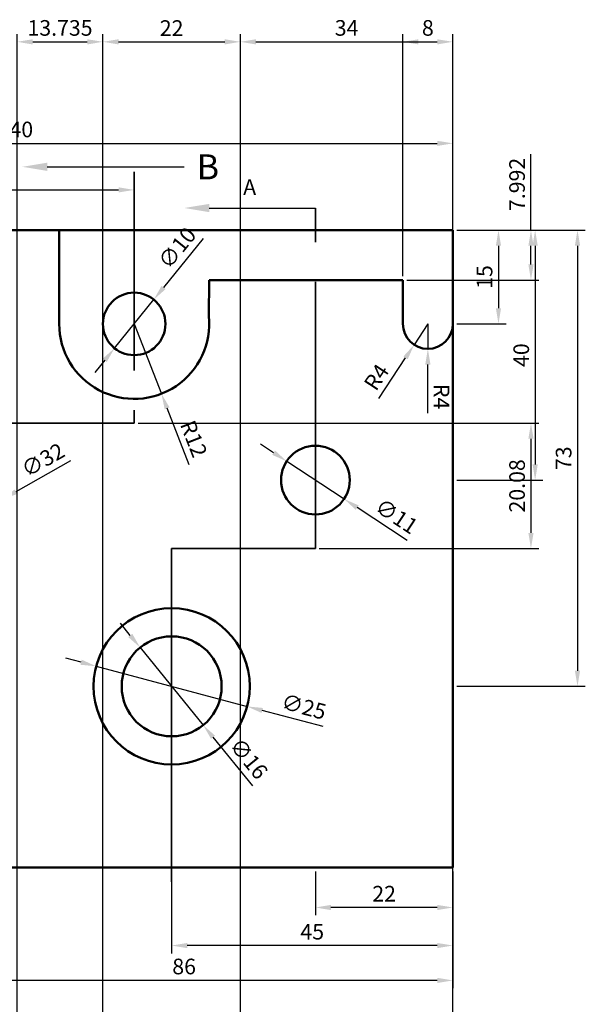
# Model space of a CAD drawing. Units: millimetres. Extents: x 2432 to 2611, y 2100 to 2357.
# Tile 3 of 3: x 2521 to 2611, y 2199 to 2357. Entities that reach past the tile are written whole.
import ezdxf
from ezdxf import colors
from ezdxf.entities.mleader import LeaderData, LeaderLine
from ezdxf.math import Vec2, Vec3

# ---------------------------------------------------------------- set-up
doc = ezdxf.new("R2010")
doc.units = ezdxf.units.MM
doc.linetypes.add('PHANTOM', pattern=[63.5, 31.75, -6.35, 6.35, -6.35, 6.35, -6.35])
for name, color, linetype, lineweight in [('M-DIMS', 2, 'Continuous', 25), ('M-OUTL', 7, 'Continuous', 50), ('M-SECT', 1, 'PHANTOM', 35), ('M-TEXT', 3, 'Continuous', 25)]:
    doc.layers.add(name, color=color, linetype=linetype, lineweight=lineweight)
doc.styles.get("Standard").update_dxf_attribs({"font": 'arial.ttf'})
doc.dimstyles.new('ISO-25', dxfattribs={"dimtxt": 2.5, "dimasz": 2.5, "dimexe": 1.25, "dimexo": 0.625, "dimtad": 1, "dimtxsty": 'Standard', "dimcen": 2.5, "dimadec": 0, "dimazin": 0, "dimtfac": 1, "dimtmove": 0, "dimatfit": 3, "dimfxl": 1, "dimarcsym": 0})

# ---------------------------------------------------------------- blocks, each defined once
blk = doc.blocks.new('*D2')
at = {"layer": 'Defpoints', "color": 0, "transparency": 16777216}
for p in [(2539.07, 2329.49), (2485.07, 2323.05), (2539.07, 2323.05)]:
    blk.add_point(p, dxfattribs=at)
at = {"layer": 'M-DIMS', "color": 0, "lineweight": -2, "transparency": 16777216}
for p, q in [((2485.07, 2323.67), (2485.07, 2330.74)), ((2539.07, 2323.67), (2539.07, 2330.74)), ((2487.57, 2329.49), (2536.57, 2329.49))]:
    blk.add_line(p, q, dxfattribs=at)
at = {"layer": 'M-DIMS', "color": 0, "transparency": 16777216}
for points in [[(2487.57, 2329.91), (2487.57, 2329.08), (2485.07, 2329.49)], [(2536.57, 2329.91), (2536.57, 2329.08), (2539.07, 2329.49)]]:
    blk.add_solid(points, dxfattribs=at)
at = {"layer": 'M-DIMS', "color": 0, "transparency": 16777216, "insert": (2512.07, 2331.39), "char_height": 2.5, "attachment_point": 5}
blk.add_mtext('54', dxfattribs=at)
blk = doc.blocks.new('*D3')
at = {"layer": 'Defpoints', "color": 0, "transparency": 16777216}
for p in [(2590.07, 2336.94), (2450.07, 2323.05), (2590.07, 2323.05)]:
    blk.add_point(p, dxfattribs=at)
at = {"layer": 'M-DIMS', "color": 0, "lineweight": -2, "transparency": 16777216}
for p, q in [((2450.07, 2323.67), (2450.07, 2338.19)), ((2452.57, 2336.94), (2587.57, 2336.94)), ((2590.07, 2323.67), (2590.07, 2338.19))]:
    blk.add_line(p, q, dxfattribs=at)
at = {"layer": 'M-DIMS', "color": 0, "transparency": 16777216}
for points in [[(2452.57, 2337.35), (2452.57, 2336.52), (2450.07, 2336.94)], [(2587.57, 2337.35), (2587.57, 2336.52), (2590.07, 2336.94)]]:
    blk.add_solid(points, dxfattribs=at)
at = {"layer": 'M-DIMS', "color": 0, "transparency": 16777216, "insert": (2520.07, 2338.84), "char_height": 2.5, "attachment_point": 5}
blk.add_mtext('140', dxfattribs=at)
blk = doc.blocks.new('*D4')
at = {"layer": 'Defpoints', "color": 0, "transparency": 16777216}
for p in [(2590.07, 2323.05), (2590.07, 2308.05), (2597.37, 2308.05)]:
    blk.add_point(p, dxfattribs=at)
at = {"layer": 'M-DIMS', "color": 0, "lineweight": -2, "transparency": 16777216}
for p, q in [((2590.7, 2323.05), (2598.62, 2323.05)), ((2597.37, 2320.55), (2597.37, 2310.55)), ((2590.7, 2308.05), (2598.62, 2308.05))]:
    blk.add_line(p, q, dxfattribs=at)
at = {"layer": 'M-DIMS', "color": 0, "transparency": 16777216}
for points in [[(2596.96, 2320.55), (2597.79, 2320.55), (2597.37, 2323.05)], [(2596.96, 2310.55), (2597.79, 2310.55), (2597.37, 2308.05)]]:
    blk.add_solid(points, dxfattribs=at)
at = {"layer": 'M-DIMS', "color": 0, "transparency": 16777216, "insert": (2595.47, 2315.55), "char_height": 2.5, "attachment_point": 5, "rotation": 90}
blk.add_mtext('15', dxfattribs=at)
blk = doc.blocks.new('*D5')
at = {"layer": 'Defpoints', "color": 0, "transparency": 16777216}
for p in [(2590.07, 2323.05), (2590.07, 2283.05), (2603.24, 2283.05)]:
    blk.add_point(p, dxfattribs=at)
at = {"layer": 'M-DIMS', "color": 0, "lineweight": -2, "transparency": 16777216}
for p, q in [((2590.7, 2323.05), (2604.49, 2323.05)), ((2603.24, 2320.55), (2603.24, 2285.55)), ((2590.7, 2283.05), (2604.49, 2283.05))]:
    blk.add_line(p, q, dxfattribs=at)
at = {"layer": 'M-DIMS', "color": 0, "transparency": 16777216}
for points in [[(2602.83, 2320.55), (2603.66, 2320.55), (2603.24, 2323.05)], [(2602.83, 2285.55), (2603.66, 2285.55), (2603.24, 2283.05)]]:
    blk.add_solid(points, dxfattribs=at)
at = {"layer": 'M-DIMS', "color": 0, "transparency": 16777216, "insert": (2601.34, 2303.05), "char_height": 2.5, "attachment_point": 5, "rotation": 90}
blk.add_mtext('40', dxfattribs=at)
blk = doc.blocks.new('*D6')
at = {"layer": 'Defpoints', "color": 0, "transparency": 16777216}
for p in [(2590.07, 2323.05), (2590.07, 2250.05), (2610.02, 2250.05)]:
    blk.add_point(p, dxfattribs=at)
at = {"layer": 'M-DIMS', "color": 0, "lineweight": -2, "transparency": 16777216}
for p, q in [((2590.7, 2323.05), (2611.27, 2323.05)), ((2610.02, 2320.55), (2610.02, 2252.55)), ((2590.7, 2250.05), (2611.27, 2250.05))]:
    blk.add_line(p, q, dxfattribs=at)
at = {"layer": 'M-DIMS', "color": 0, "transparency": 16777216}
for points in [[(2609.6, 2320.55), (2610.44, 2320.55), (2610.02, 2323.05)], [(2609.6, 2252.55), (2610.44, 2252.55), (2610.02, 2250.05)]]:
    blk.add_solid(points, dxfattribs=at)
at = {"layer": 'M-DIMS', "color": 0, "transparency": 16777216, "insert": (2608.12, 2286.55), "char_height": 2.5, "attachment_point": 5, "rotation": 90}
blk.add_mtext('73', dxfattribs=at)
blk = doc.blocks.new('*D7')
at = {"layer": 'Defpoints', "color": 0, "transparency": 16777216}
for p in [(2568.07, 2221.05), (2590.07, 2221.05), (2568.07, 2214.66)]:
    blk.add_point(p, dxfattribs=at)
at = {"layer": 'M-DIMS', "color": 0, "lineweight": -2, "transparency": 16777216}
for p, q in [((2568.07, 2220.42), (2568.07, 2213.41)), ((2590.07, 2220.42), (2590.07, 2213.41)), ((2587.57, 2214.66), (2570.57, 2214.66))]:
    blk.add_line(p, q, dxfattribs=at)
at = {"layer": 'M-DIMS', "color": 0, "transparency": 16777216}
for points in [[(2570.57, 2215.07), (2570.57, 2214.24), (2568.07, 2214.66)], [(2587.57, 2215.07), (2587.57, 2214.24), (2590.07, 2214.66)]]:
    blk.add_solid(points, dxfattribs=at)
at = {"layer": 'M-DIMS', "color": 0, "transparency": 16777216, "insert": (2579.07, 2216.54), "char_height": 2.5, "attachment_point": 5}
blk.add_mtext('22', dxfattribs=at)
blk = doc.blocks.new('*D8')
at = {"layer": 'Defpoints', "color": 0, "transparency": 16777216}
for p in [(2545.07, 2221.05), (2590.07, 2221.05), (2545.07, 2208.57)]:
    blk.add_point(p, dxfattribs=at)
at = {"layer": 'M-DIMS', "color": 0, "lineweight": -2, "transparency": 16777216}
for p, q in [((2545.07, 2220.42), (2545.07, 2207.32)), ((2590.07, 2220.42), (2590.07, 2207.32)), ((2587.57, 2208.57), (2547.57, 2208.57))]:
    blk.add_line(p, q, dxfattribs=at)
at = {"layer": 'M-DIMS', "color": 0, "transparency": 16777216}
for points in [[(2547.57, 2208.98), (2547.57, 2208.15), (2545.07, 2208.57)], [(2587.57, 2208.98), (2587.57, 2208.15), (2590.07, 2208.57)]]:
    blk.add_solid(points, dxfattribs=at)
at = {"layer": 'M-DIMS', "color": 0, "transparency": 16777216, "insert": (2567.57, 2210.46), "char_height": 2.5, "attachment_point": 5}
blk.add_mtext('45', dxfattribs=at)
blk = doc.blocks.new('*D9')
at = {"layer": 'Defpoints', "color": 0, "transparency": 16777216}
for p in [(2504.07, 2221.05), (2590.07, 2221.05), (2504.07, 2202.99)]:
    blk.add_point(p, dxfattribs=at)
at = {"layer": 'M-DIMS', "color": 0, "lineweight": -2, "transparency": 16777216}
for p, q in [((2504.07, 2220.42), (2504.07, 2201.74)), ((2590.07, 2220.42), (2590.07, 2201.74)), ((2587.57, 2202.99), (2506.57, 2202.99))]:
    blk.add_line(p, q, dxfattribs=at)
at = {"layer": 'M-DIMS', "color": 0, "transparency": 16777216}
for points in [[(2506.57, 2203.4), (2506.57, 2202.57), (2504.07, 2202.99)], [(2587.57, 2203.4), (2587.57, 2202.57), (2590.07, 2202.99)]]:
    blk.add_solid(points, dxfattribs=at)
at = {"layer": 'M-DIMS', "color": 0, "transparency": 16777216, "insert": (2547.07, 2204.89), "char_height": 2.5, "attachment_point": 5}
blk.add_mtext('86', dxfattribs=at)
blk = doc.blocks.new('*D16')
at = {"layer": 'Defpoints', "color": 0, "transparency": 16777216}
for p in [(2542.22, 2311.94), (2535.93, 2304.16)]:
    blk.add_point(p, dxfattribs=at)
at = {"layer": 'M-DIMS', "color": 0, "lineweight": -2, "transparency": 16777216}
for p, q in [((2550.1, 2321.69), (2543.79, 2313.88)), ((2535.93, 2304.16), (2542.22, 2311.94)), ((2534.36, 2302.22), (2532.79, 2300.27))]:
    blk.add_line(p, q, dxfattribs=at)
at = {"layer": 'M-DIMS', "color": 0, "transparency": 16777216}
for points in [[(2543.46, 2314.14), (2544.11, 2313.62), (2542.22, 2311.94)], [(2534.04, 2302.48), (2534.68, 2301.95), (2535.93, 2304.16)]]:
    blk.add_solid(points, dxfattribs=at)
at = {"layer": 'M-DIMS', "color": 0, "transparency": 16777216, "insert": (2546.2, 2320), "char_height": 2.5, "attachment_point": 5, "rotation": 51.0553}
blk.add_mtext('∅10', dxfattribs=at)
blk = doc.blocks.new('*D17')
at = {"layer": 'Defpoints', "color": 0, "transparency": 16777216}
for p in [(2540.03, 2256.26), (2550.12, 2243.84)]:
    blk.add_point(p, dxfattribs=at)
at = {"layer": 'M-DIMS', "color": 0, "lineweight": -2, "transparency": 16777216}
for p, q in [((2538.45, 2258.2), (2536.87, 2260.14)), ((2540.03, 2256.26), (2550.12, 2243.84)), ((2558.04, 2234.1), (2551.7, 2241.9))]:
    blk.add_line(p, q, dxfattribs=at)
at = {"layer": 'M-DIMS', "color": 0, "transparency": 16777216}
for points in [[(2538.78, 2258.46), (2538.13, 2257.93), (2540.03, 2256.26)], [(2552.02, 2242.16), (2551.37, 2241.64), (2550.12, 2243.84)]]:
    blk.add_solid(points, dxfattribs=at)
at = {"layer": 'M-DIMS', "color": 0, "transparency": 16777216, "insert": (2557.18, 2238.28), "char_height": 2.5, "attachment_point": 5, "rotation": 309.1048}
blk.add_mtext('∅16', dxfattribs=at)
blk = doc.blocks.new('*D18')
at = {"layer": 'Defpoints', "color": 0, "transparency": 16777216}
for p in [(2532.99, 2253.26), (2557.15, 2246.83)]:
    blk.add_point(p, dxfattribs=at)
at = {"layer": 'M-DIMS', "color": 0, "lineweight": -2, "transparency": 16777216}
for p, q in [((2530.58, 2253.91), (2528.16, 2254.55)), ((2532.99, 2253.26), (2557.15, 2246.83)), ((2569.3, 2243.6), (2559.57, 2246.19))]:
    blk.add_line(p, q, dxfattribs=at)
at = {"layer": 'M-DIMS', "color": 0, "transparency": 16777216}
for points in [[(2530.69, 2254.31), (2530.47, 2253.5), (2532.99, 2253.26)], [(2559.68, 2246.59), (2559.46, 2245.79), (2557.15, 2246.83)]]:
    blk.add_solid(points, dxfattribs=at)
at = {"layer": 'M-DIMS', "color": 0, "transparency": 16777216, "insert": (2566.15, 2246.48), "char_height": 2.5, "attachment_point": 5, "rotation": 345.0984}
blk.add_mtext('∅25', dxfattribs=at)
blk = doc.blocks.new('*D20')
at = {"layer": 'Defpoints', "color": 0, "transparency": 16777216}
for p in [(2517.98, 2279.96), (2490.16, 2264.14)]:
    blk.add_point(p, dxfattribs=at)
at = {"layer": 'M-DIMS', "color": 0, "lineweight": -2, "transparency": 16777216}
for p, q in [((2528.87, 2286.15), (2520.16, 2281.19)), ((2490.16, 2264.14), (2517.98, 2279.96)), ((2487.99, 2262.91), (2485.82, 2261.67))]:
    blk.add_line(p, q, dxfattribs=at)
at = {"layer": 'M-DIMS', "color": 0, "transparency": 16777216}
for points in [[(2519.95, 2281.55), (2520.36, 2280.83), (2517.98, 2279.96)], [(2487.79, 2263.27), (2488.2, 2262.54), (2490.16, 2264.14)]]:
    blk.add_solid(points, dxfattribs=at)
at = {"layer": 'M-DIMS', "color": 0, "transparency": 16777216, "insert": (2524.63, 2286), "char_height": 2.5, "attachment_point": 5, "rotation": 29.6157}
blk.add_mtext('∅32', dxfattribs=at)
blk = doc.blocks.new('*D23')
at = {"layer": 'Defpoints', "color": 0, "transparency": 16777216}
for p in [(2539.07, 2308.05), (2543.44, 2296.87)]:
    blk.add_point(p, dxfattribs=at)
at = {"layer": 'M-DIMS', "color": 0, "lineweight": -2, "transparency": 16777216}
for p, q in [((2539.07, 2308.05), (2543.44, 2296.87)), ((2547.87, 2285.51), (2544.34, 2294.54))]:
    blk.add_line(p, q, dxfattribs=at)
at = {"layer": 'M-DIMS', "color": 0, "transparency": 16777216}
blk.add_solid([(2544.73, 2294.69), (2543.96, 2294.39), (2543.44, 2296.87)], dxfattribs=at)
at = {"layer": 'M-DIMS', "color": 0, "transparency": 16777216, "insert": (2548.31, 2289.54), "char_height": 2.5, "attachment_point": 5, "rotation": 291.3135}
blk.add_mtext('R12', dxfattribs=at)
blk = doc.blocks.new('*D24')
at = {"layer": 'Defpoints', "color": 0, "transparency": 16777216}
for p in [(2586.07, 2308.05), (2583.88, 2304.71)]:
    blk.add_point(p, dxfattribs=at)
at = {"layer": 'M-DIMS', "color": 0, "lineweight": -2, "transparency": 16777216}
for p, q in [((2586.07, 2308.05), (2583.88, 2304.71)), ((2578.24, 2296.12), (2582.51, 2302.62))]:
    blk.add_line(p, q, dxfattribs=at)
at = {"layer": 'M-DIMS', "color": 0, "transparency": 16777216}
blk.add_solid([(2582.16, 2302.85), (2582.85, 2302.39), (2583.88, 2304.71)], dxfattribs=at)
at = {"layer": 'M-DIMS', "color": 0, "transparency": 16777216, "insert": (2578.12, 2299.35), "char_height": 2.5, "attachment_point": 5, "rotation": 56.6989}
blk.add_mtext('R4', dxfattribs=at)
blk = doc.blocks.new('*D25')
at = {"layer": 'Defpoints', "color": 0, "transparency": 16777216}
for p in [(2563.48, 2286.07), (2572.67, 2280.03)]:
    blk.add_point(p, dxfattribs=at)
at = {"layer": 'M-DIMS', "color": 0, "lineweight": -2, "transparency": 16777216}
for p, q in [((2561.39, 2287.44), (2559.3, 2288.81)), ((2563.48, 2286.07), (2572.67, 2280.03)), ((2582.76, 2273.41), (2574.76, 2278.66))]:
    blk.add_line(p, q, dxfattribs=at)
at = {"layer": 'M-DIMS', "color": 0, "transparency": 16777216}
for points in [[(2561.62, 2287.79), (2561.16, 2287.09), (2563.48, 2286.07)], [(2574.99, 2279.01), (2574.53, 2278.31), (2572.67, 2280.03)]]:
    blk.add_solid(points, dxfattribs=at)
at = {"layer": 'M-DIMS', "color": 0, "transparency": 16777216, "insert": (2580.89, 2277), "char_height": 2.5, "attachment_point": 5, "rotation": 326.7161}
blk.add_mtext('∅11', dxfattribs=at)
blk = doc.blocks.new('*D37')
at = {"layer": 'Defpoints', "color": 0, "transparency": 16777216}
for p in [(2590.07, 2323.05), (2602.57, 2323.05), (2582.07, 2315.06)]:
    blk.add_point(p, dxfattribs=at)
at = {"layer": 'M-DIMS', "color": 0, "lineweight": -2, "transparency": 16777216}
for p, q in [((2602.57, 2323.05), (2602.57, 2335.19)), ((2590.7, 2323.05), (2603.82, 2323.05)), ((2602.57, 2317.56), (2602.57, 2320.55)), ((2582.7, 2315.06), (2603.82, 2315.06))]:
    blk.add_line(p, q, dxfattribs=at)
at = {"layer": 'M-DIMS', "color": 0, "transparency": 16777216}
for points in [[(2602.16, 2320.55), (2602.99, 2320.55), (2602.57, 2323.05)], [(2602.16, 2317.56), (2602.99, 2317.56), (2602.57, 2315.06)]]:
    blk.add_solid(points, dxfattribs=at)
at = {"layer": 'M-DIMS', "color": 0, "transparency": 16777216, "insert": (2600.67, 2330.37), "char_height": 2.5, "attachment_point": 5, "rotation": 90}
blk.add_mtext('7.992', dxfattribs=at)
blk = doc.blocks.new('*D38')
at = {"layer": 'Defpoints', "color": 0, "transparency": 16777216}
for p in [(2590.07, 2353.19), (2590.07, 2323.05), (2582.07, 2315.06)]:
    blk.add_point(p, dxfattribs=at)
at = {"layer": 'M-DIMS', "color": 0, "lineweight": -2, "transparency": 16777216}
for p, q in [((2582.07, 2315.68), (2582.07, 2354.44)), ((2590.07, 2323.67), (2590.07, 2354.44)), ((2584.57, 2353.19), (2587.57, 2353.19))]:
    blk.add_line(p, q, dxfattribs=at)
at = {"layer": 'M-DIMS', "color": 0, "transparency": 16777216}
for points in [[(2584.57, 2353.6), (2584.57, 2352.77), (2582.07, 2353.19)], [(2587.57, 2353.6), (2587.57, 2352.77), (2590.07, 2353.19)]]:
    blk.add_solid(points, dxfattribs=at)
at = {"layer": 'M-DIMS', "color": 0, "transparency": 16777216, "insert": (2586.07, 2355.09), "char_height": 2.5, "attachment_point": 5}
blk.add_mtext('8', dxfattribs=at)
blk = doc.blocks.new('*D39')
at = {"layer": 'Defpoints', "color": 0, "transparency": 16777216}
for p in [(2539.07, 2292.17), (2568.07, 2272.09), (2602.57, 2272.09)]:
    blk.add_point(p, dxfattribs=at)
at = {"layer": 'M-DIMS', "color": 0, "lineweight": -2, "transparency": 16777216}
for p, q in [((2539.7, 2292.17), (2603.82, 2292.17)), ((2602.57, 2289.67), (2602.57, 2274.59)), ((2568.7, 2272.09), (2603.82, 2272.09))]:
    blk.add_line(p, q, dxfattribs=at)
at = {"layer": 'M-DIMS', "color": 0, "transparency": 16777216}
for points in [[(2602.16, 2289.67), (2602.99, 2289.67), (2602.57, 2292.17)], [(2602.16, 2274.59), (2602.99, 2274.59), (2602.57, 2272.09)]]:
    blk.add_solid(points, dxfattribs=at)
at = {"layer": 'M-DIMS', "color": 0, "transparency": 16777216, "insert": (2600.67, 2282.13), "char_height": 2.5, "attachment_point": 5, "rotation": 90}
blk.add_mtext('20.08', dxfattribs=at)
blk = doc.blocks.new('*D45')
at = {"layer": 'Defpoints', "color": 0, "transparency": 16777216}
for p in [(2534.07, 2353.19), (2534.07, 2151.26), (2520.34, 2145.26)]:
    blk.add_point(p, dxfattribs=at)
at = {"layer": 'M-DIMS', "color": 0, "lineweight": -2, "transparency": 16777216}
for p, q in [((2520.34, 2145.89), (2520.34, 2354.44)), ((2534.07, 2151.89), (2534.07, 2354.44)), ((2522.84, 2353.19), (2531.57, 2353.19))]:
    blk.add_line(p, q, dxfattribs=at)
at = {"layer": 'M-DIMS', "color": 0, "transparency": 16777216}
for points in [[(2522.84, 2353.6), (2522.84, 2352.77), (2520.34, 2353.19)], [(2531.57, 2353.6), (2531.57, 2352.77), (2534.07, 2353.19)]]:
    blk.add_solid(points, dxfattribs=at)
at = {"layer": 'M-DIMS', "color": 0, "transparency": 16777216, "insert": (2527.21, 2355.09), "char_height": 2.5, "attachment_point": 5}
blk.add_mtext('13.735', dxfattribs=at)
blk = doc.blocks.new('*D46')
at = {"layer": 'Defpoints', "color": 0, "transparency": 16777216}
for p in [(2556.07, 2353.19), (2534.07, 2151.26), (2556.07, 2151.26)]:
    blk.add_point(p, dxfattribs=at)
at = {"layer": 'M-DIMS', "color": 0, "lineweight": -2, "transparency": 16777216}
for p, q in [((2534.07, 2151.89), (2534.07, 2354.44)), ((2556.07, 2151.89), (2556.07, 2354.44)), ((2536.57, 2353.19), (2553.57, 2353.19))]:
    blk.add_line(p, q, dxfattribs=at)
at = {"layer": 'M-DIMS', "color": 0, "transparency": 16777216}
for points in [[(2536.57, 2353.6), (2536.57, 2352.77), (2534.07, 2353.19)], [(2553.57, 2353.6), (2553.57, 2352.77), (2556.07, 2353.19)]]:
    blk.add_solid(points, dxfattribs=at)
at = {"layer": 'M-DIMS', "color": 0, "transparency": 16777216, "insert": (2545.07, 2355.07), "char_height": 2.5, "attachment_point": 5}
blk.add_mtext('22', dxfattribs=at)
blk = doc.blocks.new('*D47')
at = {"layer": 'Defpoints', "color": 0, "transparency": 16777216}
for p in [(2590.07, 2353.19), (2556.07, 2151.26), (2590.07, 2151.26)]:
    blk.add_point(p, dxfattribs=at)
at = {"layer": 'M-DIMS', "color": 0, "lineweight": -2, "transparency": 16777216}
for p, q in [((2556.07, 2151.89), (2556.07, 2354.44)), ((2590.07, 2151.89), (2590.07, 2354.44)), ((2558.57, 2353.19), (2587.57, 2353.19))]:
    blk.add_line(p, q, dxfattribs=at)
at = {"layer": 'M-DIMS', "color": 0, "transparency": 16777216}
for points in [[(2558.57, 2353.6), (2558.57, 2352.77), (2556.07, 2353.19)], [(2587.57, 2353.6), (2587.57, 2352.77), (2590.07, 2353.19)]]:
    blk.add_solid(points, dxfattribs=at)
at = {"layer": 'M-DIMS', "color": 0, "transparency": 16777216, "insert": (2573.07, 2355.09), "char_height": 2.5, "attachment_point": 5}
blk.add_mtext('34', dxfattribs=at)
blk = doc.blocks.new('*D54')
at = {"layer": 'Defpoints', "color": 0, "transparency": 16777216}
for p in [(2586.07, 2308.05), (2586.07, 2304.05)]:
    blk.add_point(p, dxfattribs=at)
at = {"layer": 'M-DIMS', "color": 0, "lineweight": -2, "transparency": 16777216}
for p, q in [((2586.07, 2308.05), (2586.07, 2304.05)), ((2586.08, 2293.78), (2586.08, 2301.55))]:
    blk.add_line(p, q, dxfattribs=at)
at = {"layer": 'M-DIMS', "color": 0, "transparency": 16777216}
blk.add_solid([(2586.49, 2301.55), (2585.66, 2301.55), (2586.07, 2304.05)], dxfattribs=at)
at = {"layer": 'M-DIMS', "color": 0, "transparency": 16777216, "insert": (2587.95, 2296.41), "char_height": 2.5, "attachment_point": 5, "rotation": 270.0065}
blk.add_mtext('R4', dxfattribs=at)

msp = doc.modelspace()

# ---------------------------------------------------------------- linework, layer by layer
at = {"layer": 'M-OUTL'}
for p, q in [((2450.0745, 2323.0493), (2590.0745, 2323.0493)), ((2527.0745, 2308.0493), (2527.0745, 2323.0493)), ((2590.0745, 2323.0493), (2590.0745, 2221.0493)), ((2590.0745, 2323.0493), (2590.0745, 2308.0493)), ((2590.0745, 2323.0493), (2590.0745, 2283.0493)), ((2551.0745, 2315.057), (2551.0083, 2309.3087)), ((2551.0745, 2315.057), (2582.0745, 2315.057)), ((2582.0745, 2308.0493), (2582.0745, 2315.057)), ((2590.0745, 2221.0493), (2450.0745, 2221.0493))]:
    msp.add_line(p, q, dxfattribs=at)
for centre, radius in [((2539.0745, 2308.0493), 5), ((2568.0745, 2283.0493), 5.5), ((2545.0745, 2250.0493), 12.5), ((2545.0745, 2250.0493), 8)]:
    msp.add_circle(centre, radius, dxfattribs=at)
for centre, radius, end in [((2539.0745, 2308.0493), 12, 6.024376), ((2586.0745, 2308.0493), 4, 0)]:
    msp.add_arc(centre, radius, 180, end, dxfattribs=at)
at = {"layer": 'M-SECT'}
for p, q in [((2539.0745, 2308.0493), (2539.0745, 2332.3604)), ((2539.0745, 2332.3604), (2539.0745, 2292.1705)), ((2568.0745, 2323.0493), (2568.0745, 2326.5944)), ((2568.0745, 2283.0493), (2568.0745, 2323.0493)), ((2539.0745, 2292.1705), (2511.6649, 2292.1705)), ((2568.0745, 2283.0493), (2568.0745, 2272.0921)), ((2545.0745, 2250.0493), (2545.0745, 2272.0921)), ((2568.0745, 2272.0921), (2545.0745, 2272.0921)), ((2568.0745, 2272.0921), (2548.1371, 2272.0921)), ((2545.0745, 2250.5245), (2545.0745, 2213.8698))]:
    msp.add_line(p, q, dxfattribs=at)

# ---------------------------------------------------------------- texts
at = {"layer": 'M-TEXT', "insert": (2556.5179, 2331.1874), "char_height": 2.5, "attachment_point": 1}
msp.add_mtext_dynamic_manual_height_columns('A', width=11.503363, gutter_width=12.5, heights=[0], dxfattribs=at)

# ---------------------------------------------------------------- dimensions: what is measured, and where the dimension line sits
at = {"layer": 'M-DIMS'}
for base, p1, p2, override, picture, middle in [((2534.0745, 2353.1874), (2520.3395, 2145.2616), (2534.0745, 2151.2616), {"dimdec": 3, "dimlfac": 1, "dimrnd": 0, "dimzin": 0, "dimdsep": 46, "dimlunit": 2}, '*D45', (2527.207, 2355.0897)), ((2556.0745, 2353.1874), (2534.0745, 2151.2616), (2556.0745, 2151.2616), {"dimdec": 0, "dimlfac": 1, "dimrnd": 0, "dimzin": 0, "dimdsep": 46, "dimlunit": 2}, '*D46', (2545.0745, 2355.0676)), ((2590.0745, 2353.1874), (2556.0745, 2151.2616), (2590.0745, 2151.2616), {"dimdec": 0, "dimlfac": 1, "dimrnd": 0, "dimzin": 0, "dimdsep": 46, "dimlunit": 2}, '*D47', (2573.0745, 2355.0897)), ((2590.0745, 2353.1874), (2582.0745, 2315.057), (2590.0745, 2323.0493), {"dimdec": 0, "dimlfac": 1, "dimrnd": 0, "dimzin": 0, "dimdsep": 46, "dimlunit": 2}, '*D38', (2586.0745, 2355.0889)), ((2590.0745, 2336.9374), (2450.0745, 2323.0493), (2590.0745, 2323.0493), {"dimclrd": 0, "dimclre": 0, "dimclrt": 0}, '*D3', (2520.0745, 2338.8389)), ((2539.0745, 2329.4923), (2485.0745, 2323.0493), (2539.0745, 2323.0493), {"dimclrd": 0, "dimclre": 0, "dimclrt": 0}, '*D2', (2512.0745, 2331.3886)), ((2504.0745, 2202.9855), (2590.0745, 2221.0493), (2504.0745, 2221.0493), {"dimclrd": 0, "dimclre": 0, "dimclrt": 0}, '*D9', (2547.0745, 2204.8869)), ((2545.0745, 2208.5652), (2590.0745, 2221.0493), (2545.0745, 2221.0493), {"dimclrd": 0, "dimclre": 0, "dimclrt": 0}, '*D8', (2567.5745, 2210.4616)), ((2568.0745, 2214.6567), (2590.0745, 2221.0493), (2568.0745, 2221.0493), {"dimclrd": 0, "dimclre": 0, "dimclrt": 0}, '*D7', (2579.0745, 2216.5368))]:
    dim = msp.add_linear_dim(base=base, p1=p1, p2=p2, dimstyle='ISO-25', override=override, dxfattribs=at)
    dim.commit()
    dim.dimension.update_dxf_attribs({"geometry": picture, "text_midpoint": middle})
for base, p1, p2, override, picture, middle in [((2602.5745, 2323.0493), (2582.0745, 2315.057), (2590.0745, 2323.0493), {"dimdec": 3, "dimlfac": 1, "dimrnd": 0, "dimzin": 0, "dimdsep": 46, "dimlunit": 2}, '*D37', (2600.6731, 2330.3694)), ((2597.3735, 2308.0493), (2590.0745, 2323.0493), (2590.0745, 2308.0493), {"dimclrd": 0, "dimclre": 0, "dimclrt": 0}, '*D4', (2595.4721, 2315.5493)), ((2603.2444, 2283.0493), (2590.0745, 2323.0493), (2590.0745, 2283.0493), {"dimclrd": 0, "dimclre": 0, "dimclrt": 0}, '*D5', (2601.343, 2303.0493)), ((2610.0186, 2250.0493), (2590.0745, 2323.0493), (2590.0745, 2250.0493), {"dimclrd": 0, "dimclre": 0, "dimclrt": 0}, '*D6', (2608.1163, 2286.5493)), ((2602.5745, 2272.0921), (2539.0745, 2292.1705), (2568.0745, 2272.0921), {"dimdec": 2, "dimlfac": 1, "dimrnd": 0, "dimzin": 0, "dimdsep": 46, "dimlunit": 2}, '*D39', (2600.6731, 2282.1313))]:
    dim = msp.add_linear_dim(base=base, p1=p1, p2=p2, angle=90, dimstyle='ISO-25', override=override, dxfattribs=at)
    dim.commit()
    dim.dimension.update_dxf_attribs({"geometry": picture, "text_midpoint": middle})
for p1, p2, picture, middle in [((2535.9317, 2304.1606), (2542.2174, 2311.9381), '*D16', (2546.1976, 2319.9991)), ((2490.1648, 2264.1424), (2517.9843, 2279.9562), '*D20', (2524.6281, 2286.0004)), ((2563.4768, 2286.0677), (2572.6723, 2280.031), '*D25', (2580.8885, 2276.9954)), ((2540.0286, 2256.2573), (2550.1205, 2243.8414), '*D17', (2557.1848, 2238.2756)), ((2532.9949, 2253.2638), (2557.1542, 2246.8348), '*D18', (2566.1506, 2246.4807))]:
    dim = msp.add_diameter_dim_2p(p1=p1, p2=p2, dimstyle='ISO-25', override={"dimclrd": 0, "dimclre": 0, "dimclrt": 0}, dxfattribs=at)
    dim.commit()
    dim.dimension.update_dxf_attribs({"geometry": picture, "text_midpoint": middle})
for center, mpoint, override, picture, middle in [((2539.0745, 2308.0493), (2543.4362, 2296.87), {"dimclrd": 0, "dimclre": 0, "dimclrt": 0}, '*D23', (2548.3132, 2289.5425)), ((2586.0745, 2308.0493), (2583.8784, 2304.7061), {"dimclrd": 0, "dimclre": 0, "dimclrt": 0}, '*D24', (2578.119, 2299.3538)), ((2586.0745, 2308.0493), (2586.075, 2304.0493), {"dimdec": 0, "dimlfac": 1, "dimrnd": 0, "dimzin": 0, "dimdsep": 46, "dimlunit": 2}, '*D54', (2587.9509, 2296.414))]:
    dim = msp.add_radius_dim(center=center, mpoint=mpoint, dimstyle='ISO-25', override=override, dxfattribs=at)
    dim.commit()
    dim.dimension.update_dxf_attribs({"geometry": picture, "text_midpoint": middle})

# ---------------------------------------------------------------- leaders
at = {"layer": 'M-TEXT'}
ml = msp.add_multileader_mtext('Standard', dxfattribs=at)
ml.set_content('B', color=256)
ml.set_leader_properties()
ml.build(insert=Vec2(0, 0))
ctx = ml.context
ctx.base_point, ctx.plane_origin = Vec3(2547.0745, 2333.1874), Vec3(2521.1721, 2333.1874)
notes = []
notes.append((ctx, [(0, (1, 1, 0), (2539.0745, 2333.1874), (1, 0), 8, [(0, [(2521.1721, 2333.1874)], 0, [])])]))
ctx.mtext.insert, ctx.mtext.flow_direction = Vec3(2549.0745, 2335.1874), 5
ml = msp.add_multileader_mtext('Standard', dxfattribs=at)
ml.set_content('', color=256)
ml.set_leader_properties()
ml.build(insert=Vec2(0, 0))
ctx = ml.context
ctx.base_point, ctx.plane_origin = Vec3(2568.0745, 2326.5944), Vec3(2547.085, 2326.5944)
notes.append((ctx, [(0, (1, 1, 0), (2560.0745, 2326.5944), (1, 0), 8, [(0, [(2547.085, 2326.5944)], 0, [])])]))
ctx.mtext.insert, ctx.mtext.flow_direction = Vec3(2570.0745, 2328.5944), 5
for ctx, leaders in notes:
    for number, flags, end, landing, length, lines in leaders:
        leader = LeaderData()
        leader.index, (leader.has_last_leader_line, leader.has_dogleg_vector, leader.attachment_direction) = number, flags
        leader.last_leader_point, leader.dogleg_vector, leader.dogleg_length = Vec3(end), Vec3(landing), length
        for number, points, colour, breaks in lines:
            line = LeaderLine()
            line.index, line.vertices, line.color, line.breaks = number, Vec3.list(points), colors.encode_raw_color(colour), breaks
            leader.lines.append(line)
        ctx.leaders.append(leader)

doc.saveas('drawing.dxf')
